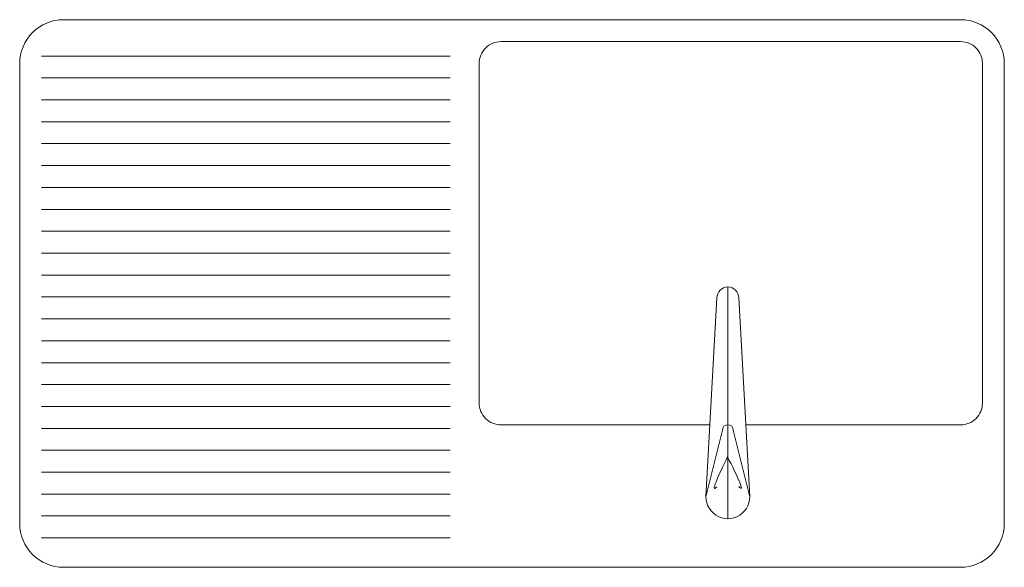
# Model space of a CAD drawing. Units: inches. Extents: x 3064 to 19385, y 846 to 15425.
# Tile 108 of 108: x 18485 to 19385, y 14925 to 15425. Entities that reach past the tile are written whole.
import ezdxf

# ---------------------------------------------------------------- set-up
doc = ezdxf.new("R2010")
doc.units = ezdxf.units.IN
doc.layers.add('A-FLOR-FIXT', color=9, linetype='Continuous', lineweight=18)

# ---------------------------------------------------------------- blocks, each defined once
blk = doc.blocks.new('SINK90X50')
for p, q in [((-56.58, 553.17), (-430, 553.17)), ((-56.58, 533.17), (-430, 533.17)), ((197.31, 535.61), (197.31, 324.05)), ((-56.58, 513.17), (-430, 513.17)), ((192.31, 454.83), (177.31, 515.61)), ((187.31, 334.05), (177.31, 515.61)), ((202.31, 454.83), (217.31, 515.61)), ((207.31, 334.05), (217.31, 515.61)), ((-56.58, 493.17), (-430, 493.17)), ((-56.58, 473.17), (-430, 473.17)), ((-56.58, 453.17), (-430, 453.17)), ((-56.58, 433.17), (-430, 433.17)), ((-56.58, 413.17), (-430, 413.17)), ((-56.58, 393.17), (-430, 393.17)), ((-56.58, 373.17), (-430, 373.17)), ((-56.58, 353.17), (-430, 353.17)), ((-56.58, 333.17), (-430, 333.17)), ((-56.58, 313.17), (-430, 313.17)), ((-56.58, 293.17), (-430, 293.17)), ((-56.58, 273.17), (-430, 273.17)), ((-56.58, 253.17), (-430, 253.17)), ((-56.58, 233.17), (-430, 233.17)), ((-56.58, 213.17), (-430, 213.17)), ((-56.58, 193.17), (-430, 193.17)), ((-56.58, 173.17), (-430, 173.17)), ((-56.58, 153.17), (-430, 153.17)), ((-56.58, 133.17), (-430, 133.17)), ((-56.58, 113.17), (-430, 113.17))]:
    blk.add_line(p, q)
blk.add_lwpolyline([(450, 540, 0.414214), (410, 580), (-410, 580, 0.414214), (-450, 540), (-450, 120, 0.414214), (-410, 80), (410, 80, 0.414214), (450, 120)], format="xyb", close=True)
blk.add_lwpolyline([(180.93, 450), (-10, 450, 0.414214), (-30, 430), (-30, 120, 0.414214), (-10, 100), (410, 100, 0.414214), (430, 120), (430, 430, 0.414214), (410, 450), (213.7, 450)], format="xyb")
for centre, radius, start, end in [((197.31, 515.61), 20, 351.30616, 188.69384), ((197.31, 454.83), 5, 180, 0), ((197.31, 334.05), 10, 180, 0)]:
    blk.add_arc(centre, radius, start, end)
for points in [[(187.22, 506.4), (180.63, 513.42), (188.84, 496.32), (197.05, 479.21)], [(207.27, 506.25), (213.96, 513.18), (205.51, 496.2), (197.05, 479.21)]]:
    blk.add_open_spline(points, degree=3)

msp = doc.modelspace()

# ---------------------------------------------------------------- block references
at = {"layer": 'A-FLOR-FIXT', "yscale": -1}
msp.add_blockref('SINK90X50', (18934.58, 15504.75), dxfattribs=at)

doc.saveas('drawing.dxf')
